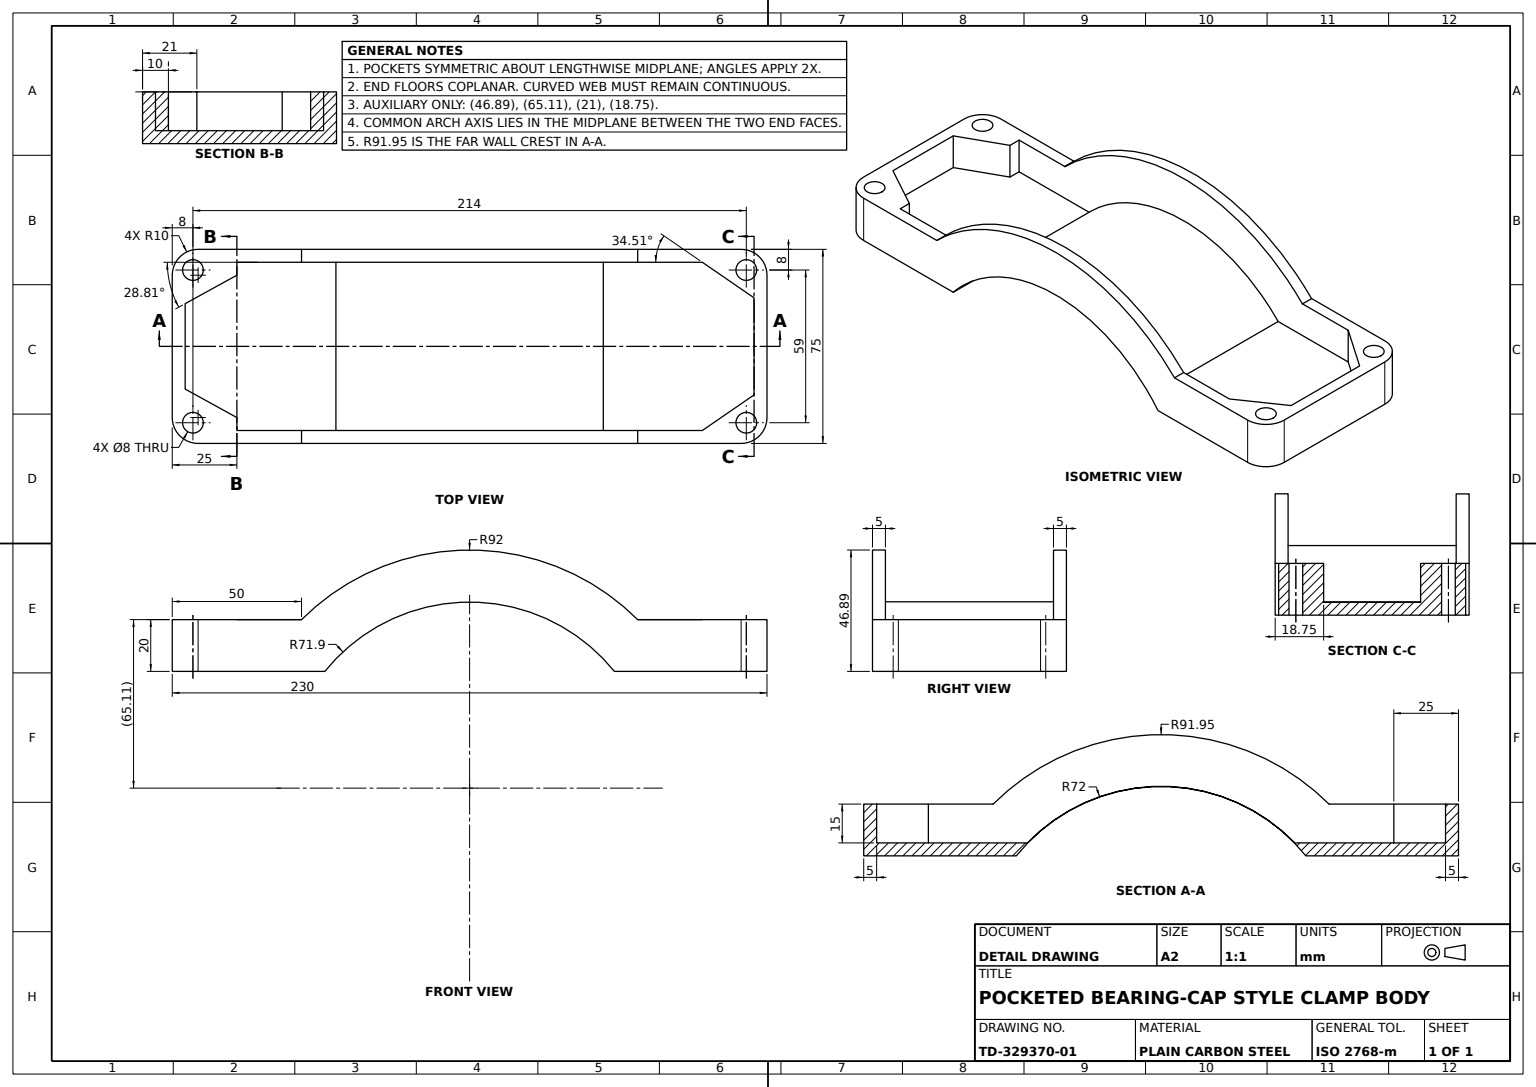
SolidWorks part; units mm, degrees
material "Plain Carbon Steel"
ref_plane "Front Plane" through (0, 0, 0) normal (0, 0, 1) x (1, 0, 0)
ref_plane "Top Plane" through (0, 0, 0) normal (0, 1, 0) x (1, 0, 0)
ref_plane "Right Plane" through (0, 0, 0) normal (1, 0, 0) x (0, 0, -1)
sketch "Side Wall Profile Sketch" plane through (0, 0, 0) normal (1, 0, 0) x (0, 0, -1)
  line L4 (65, 65.1076) -> (115, 65.1076)
  line L5 (115, 65.1076) -> (115, 45.1076)
  line L6 (95, 45.1076) -> (95, 45.1076)
  line L7 (56.1187, 45.1076) -> (95, 45.1076)
  line L8 (95, 45.1076) -> (115, 45.1076)
  line L9 (-65, 65.1076) -> (-115, 65.1076)
  line L10 (-115, 65.1076) -> (-115, 45.1076)
  line L11 (-115, 45.1076) -> (-56.1187, 45.1076)
  arc A0 (65, 65.1076) -> (-65, 65.1076) centre (0, 0) ccw
  arc A1 (56.1187, 45.1076) -> (-56.1187, 45.1076) centre (0, 0) ccw
  arc A2 (56.1187, 45.1076) -> (-50.8696, 50.9538) centre (0, 0) ccw construction
  dimension "D1" = 92
  dimension "D2" = 50
  dimension "D3" = 65.1076
  dimension "D5" = 50
  dimension "D6" = 20
  dimension "D7" = 65.1076
  dimension "D4" = 20
extrude "Side Wall" add sketch "Side Wall Profile Sketch" against normal blind 5 contours A1 L7 L8 L5 L4 A0 L9 L10 L11
sketch "End Flange A Sketch" plane through (0, 0, 115) normal (0, 0, 1) x (1, 0, 0)
  line L0 (0, 45.1076) -> (-75, 45.1076)
  line L1 (-75, 45.1076) -> (-75, 65.1076)
  line L2 (-75, 65.1076) -> (-5, 65.1076)
  line L3 (-5, 65.1076) -> (0, 65.1076)
  line L4 (0, 65.1076) -> (0, 45.1076)
  line L5 (0, 65.1076) -> (0, 45.1076) construction
  dimension "D1" = 75
extrude "End Flange A" add sketch "End Flange A Sketch" against normal blind 50
sketch "Flange A Pocket Sketch" plane through (0, 65.1076, 0) normal (0, 1, 0) x (1, 0, 0)
  line L1 (0, -65) -> (0, -115) construction
  line L2 (-5, -90) -> (-10, -90)
  line L3 (-70, -110) -> (-54, -110)
  line L5 (-21, -110) -> (-5, -110)
  line L6 (-21, -110) -> (-10, -90)
  line L9 (-70, -90) -> (-65, -90)
  line L10 (-65, -90) -> (-54, -110)
  line L13 (-70, -90) -> (-70, -110)
  line L14 (-5, -90) -> (-5, -110)
  line L17 (-70, -90) -> (-70, -65)
  line L18 (-5, -65) -> (-75, -65) construction
  line L19 (-70, -65) -> (-5, -65)
  line L20 (-5, 65) -> (-5, -65) construction
  line L21 (-5, -65) -> (-5, -90)
  line L23 (-54, -110) -> (-21, -110)
  line M9 (-5, -65) -> (-75, -65)
  dimension "D1" = 10
  dimension "D2" = 21
  dimension "D3" = 54
  dimension "D4" = 25
  dimension "D5" = 45
extrude "Flange A Pocket" cut sketch "Flange A Pocket Sketch" against normal blind 15 contours L10 L23 L6 L2 L21 L17 L9 M9
sketch "Arch Shell Sketch" plane through (0, 0, 0) normal (1, 0, 0) x (0, 0, -1)
  line L0 (-56.1187, 45.1076) -> (-55.9862, 45.1076)
  line L1 (55.9862, 45.1076) -> (56.1187, 45.1076)
  line L8 (-65, 65.1076) -> (-115, 65.1076)
  line L9 (-115, 65.1076) -> (-115, 45.1076)
  line L10 (-115, 45.1076) -> (-56.1187, 45.1076)
  line L11 (56.1187, 45.1076) -> (115, 45.1076)
  line L12 (115, 45.1076) -> (115, 65.1076)
  line L13 (115, 65.1076) -> (65, 65.1076)
  arc A0 (55.9862, 45.1076) -> (-55.9862, 45.1076) centre (0, 0) ccw
  arc A3 (65, 65.1076) -> (-65, 65.1076) centre (0, 0) ccw
  arc A4 (56.1187, 45.1076) -> (-56.1187, 45.1076) centre (0, 0) ccw
  arc A6 (56.1187, 45.1076) -> (-56.1187, 45.1076) centre (0, 0) ccw
  dimension "D2" = 71.8968
  dimension "D1" = 0
extrude "Arch Shell" add sketch "Arch Shell Sketch" against normal blind 75
sketch "Side Wall Extension Sketch" plane through (-75, 0, 0) normal (-1, 0, 0) x (0, 0, 1)
  line L0 (-80.1312, 45.1076) -> (-56.1187, 45.1076)
  line L1 (-56.1187, 45.1076) -> (-115, 45.1076) construction
  line L2 (65, 45.1076) -> (115, 45.1076) construction
  line L3 (56.1187, 45.1076) -> (80.1312, 45.1076)
  line L4 (65, 65.1076) -> (65, 45.1076)
  line L5 (-65, 65.1076) -> (-65, 65.0438)
  line L6 (-65, 45.1076) -> (-56.1187, 45.1076)
  arc A0 (65, 65.0438) -> (-80.1312, 45.1076) centre (0, 0) ccw
  arc A1 (56.1187, 45.1076) -> (-56.1187, 45.1076) centre (0, 0) ccw
  dimension "D1" = 91.9549
  dimension "D2" = 72
extrude "Side Wall Extension" add sketch "Side Wall Extension Sketch" against normal blind 5 contours A1 L3 L4 A0 L0
sketch "Flange A Rim Sketch" plane through (-75, 0, 0) normal (-1, 0, 0) x (0, 0, 1)
  line L0 (55.9862, 45.1076) -> (65, 45.1076)
  line L1 (65, 45.1076) -> (65, 50.1076)
  line L2 (65, 50.1076) -> (51.5595, 50.1076)
  line L3 (65, 65.1076) -> (65, 65.0438) construction
  arc A0 (55.9862, 45.1076) -> (-55.9862, 45.1076) centre (0, 0) ccw construction
  arc A1 (55.9862, 45.1076) -> (51.5595, 50.1076) centre (0, 0) ccw
  dimension "D1" = 13.4405
extrude "Flange A Rim" add sketch "Flange A Rim Sketch" against normal blind 75
sketch "End Flange B Sketch" plane through (0, 0, -115) normal (0, 0, -1) x (-1, 0, 0)
  line L0 (0, 45.1076) -> (75, 45.1076)
  line L1 (75, 45.1076) -> (75, 65.1076)
  line L2 (75, 45.1076) -> (75, 91.9549) construction
  line L3 (75, 65.1076) -> (0, 65.1076)
  line L4 (0, 65.1076) -> (0, 45.1076)
extrude "End Flange B" add sketch "End Flange B Sketch" against normal blind 50
sketch "Flange B Pocket Sketch" plane through (0, 65.1076, 0) normal (0, 1, 0) x (1, 0, 0)
  line L0 (-70, 90) -> (-70, 65)
  line L1 (-75, 115) -> (0, 115) construction
  line L2 (-37.5, 110) -> (-18.75, 110)
  line L3 (-37.5, 110) -> (-56.25, 110)
  line L5 (-75, 115) -> (-75, 90)
  line L6 (-75, 65) -> (-75, 115) construction
  line L7 (-75, 90) -> (-70, 90)
  line L8 (-70, 90) -> (-56.25, 110)
  line L9 (0, 115) -> (0, 90)
  line L10 (0, 65) -> (0, 115) construction
  line L11 (0, 90) -> (-5, 90)
  line L12 (-5, 90) -> (-18.75, 110)
  line L13 (-75, 115) -> (0, 115)
  line L14 (-75, 65) -> (-5, 65) construction
  line L15 (-70, 65) -> (-5, 65)
  line L16 (-5, 65) -> (-5, 90)
  line M14 (-75, 65) -> (-5, 65)
  dimension "D1" = 18.75
  dimension "D2" = 5
extrude "Flange B Pocket" cut sketch "Flange B Pocket Sketch" against normal blind 15 contours L16 L12 L2 L3 L8 L0 M14
sketch "Flange B Rim Sketch" plane through (0, 0, 0) normal (1, 0, 0) x (0, 0, -1)
  line L0 (65, 45.1076) -> (65, 50.1076)
  line L1 (65, 50.1076) -> (51.5595, 50.1076)
  line L2 (55.9862, 45.1076) -> (65, 45.1076)
  arc A0 (55.9862, 45.1076) -> (-55.9862, 45.1076) centre (0, 0) ccw construction
  arc A1 (51.5595, 50.1076) -> (55.9862, 45.1076) centre (0, 0) cw
  dimension "D1" = 116.5595
extrude "Flange B Rim" add sketch "Flange B Rim Sketch" against normal blind 75
sketch "Bolt Holes Sketch" plane through (0, 65.1076, 0) normal (0, 1, 0) x (1, 0, 0)
  line L0 (-70, 90) -> (-70, 65) construction
  line L1 (-56.25, 110) -> (-18.75, 110) construction
  circle A0 centre (-8, 107) radius 4
  circle A1 centre (-67, 107) radius 4
  circle A2 centre (-8, -107) radius 4
  circle A3 centre (-67, -107) radius 4
  dimension "D1" = 8
  dimension "D2" = 3
  dimension "D3" = 62
  dimension "D4" = 3
  dimension "D5" = 217
extrude "Bolt Holes 4x" cut sketch "Bolt Holes Sketch" against normal blind 75
fillet "Corner Fillets R10 A" radius 10 1 edges at (0, 55.1076, 115)
fillet "Corner Fillets R10 B" radius 10 1 edges at (-75, 55.1076, 115)
fillet "Corner Fillets R10 C" radius 10 1 edges at (-75, 55.1076, -115)
fillet "Corner Fillets R10 D" radius 10 1 edges at (0, 55.1076, -115)
